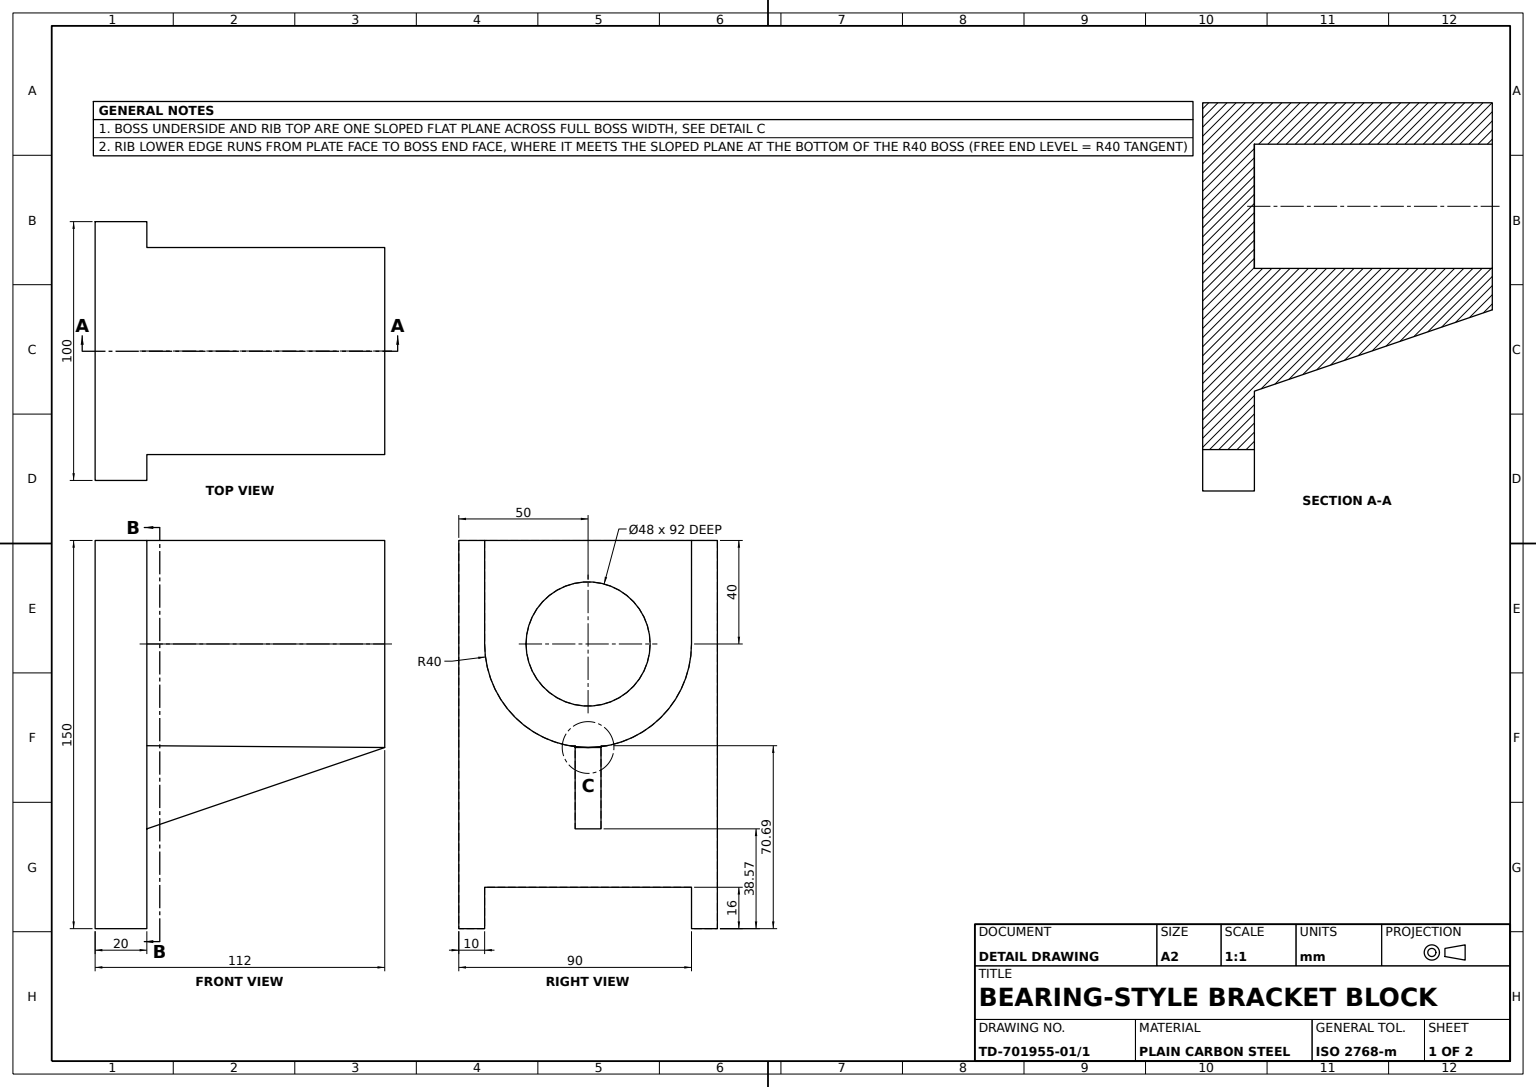
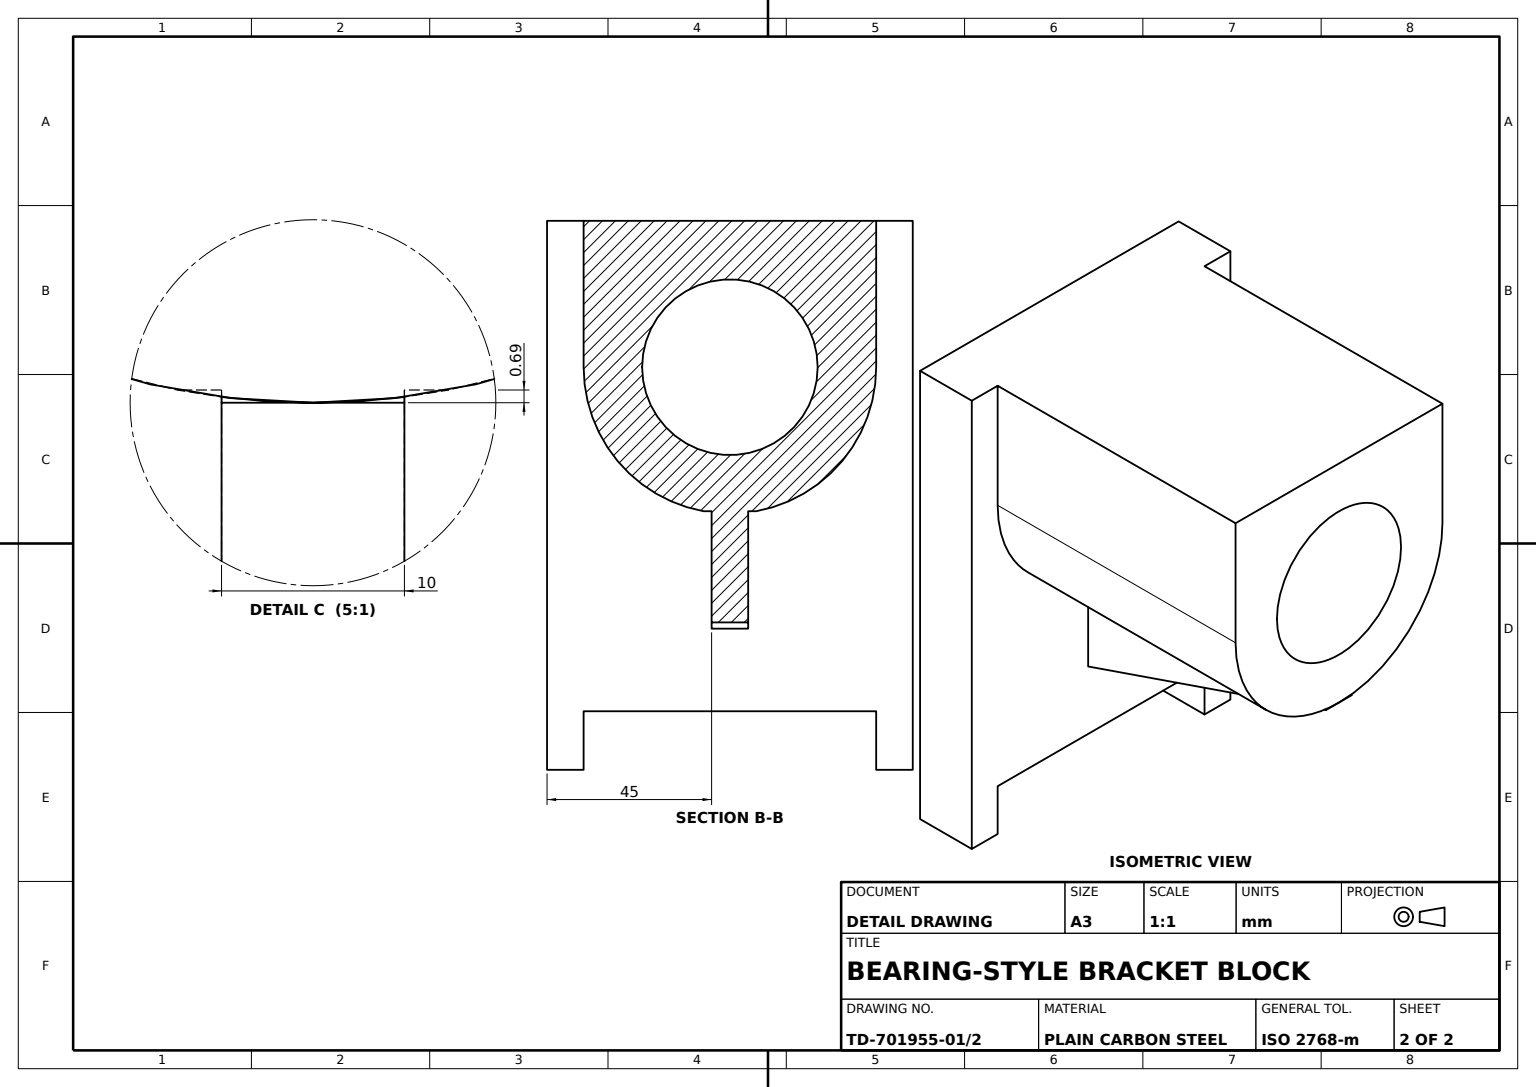
from build123d import *

# Parameters (mm, degrees)
BASE_PLATE_20MM_DEPTH   = 20
BLOCK_92MM_DEPTH        = 92
RELIEF_CUT_SKETCH_R     = 24
RELIEF_CUT_DEPTH        = 92
GUSSET_100MM_DEPTH      = 100
GUSSET_TRIM_CUT_1_DEPTH = 45
GUSSET_TRIM_CUT_2_DEPTH = 45


with BuildPart() as part:
    # Base Plate Sketch → Base Plate 20mm (new body)
    with BuildSketch(Plane.XY):
        Polygon((0, 0), (100, 0), (100, -150), (90, -150), (90, -134), (10, -134), (10, -150), (0, -150), align=None)
    extrude(amount=BASE_PLATE_20MM_DEPTH)

    # Block Sketch → Block 92mm (add)
    with BuildSketch(Plane(origin=(0, 0, 0), x_dir=(-1, 0, 0), z_dir=(0, 0, -1))):
        with BuildLine():
            Line((-10, -40), (-10, 0))
            Line((-10, 0), (-90, 0))
            Line((-90, 0), (-90, -40))
            ThreePointArc((-90, -40), (-50, -80), (-10, -40))
        make_face()
    extrude(amount=BLOCK_92MM_DEPTH)

    # Relief Cut Sketch → Relief Cut (cut)
    with BuildSketch(Plane(origin=(0, 0, -92), x_dir=(-1, 0, 0), z_dir=(0, 0, -1))):
        with Locations((-50, -40)):
            Circle(RELIEF_CUT_SKETCH_R)
    extrude(amount=-RELIEF_CUT_DEPTH, mode=Mode.SUBTRACT)

    # Gusset Sketch → Gusset 100mm (add)
    with BuildSketch(Plane.ZY):
        Polygon((-92, -80), (0, -111.42938948), (0, -79.30503211), align=None)
    extrude(amount=-GUSSET_100MM_DEPTH)

    # Gusset Trim Sketch 1 → Gusset Trim Cut 1 (cut)
    with BuildSketch(Plane.ZY):
        Polygon((-92, -80), (0, -79.30503211), (0, -111.42938948), align=None)
    extrude(amount=-GUSSET_TRIM_CUT_1_DEPTH, mode=Mode.SUBTRACT)

    # Gusset Trim Sketch 2 → Gusset Trim Cut 2 (cut)
    with BuildSketch(Plane(origin=(100, 0, 0), x_dir=(0, 0, -1), z_dir=(1, 0, 0))):
        Polygon((0, -79.30503211), (92, -80), (0, -111.42938948), align=None)
    extrude(amount=-GUSSET_TRIM_CUT_2_DEPTH, mode=Mode.SUBTRACT)


solid = part.part
